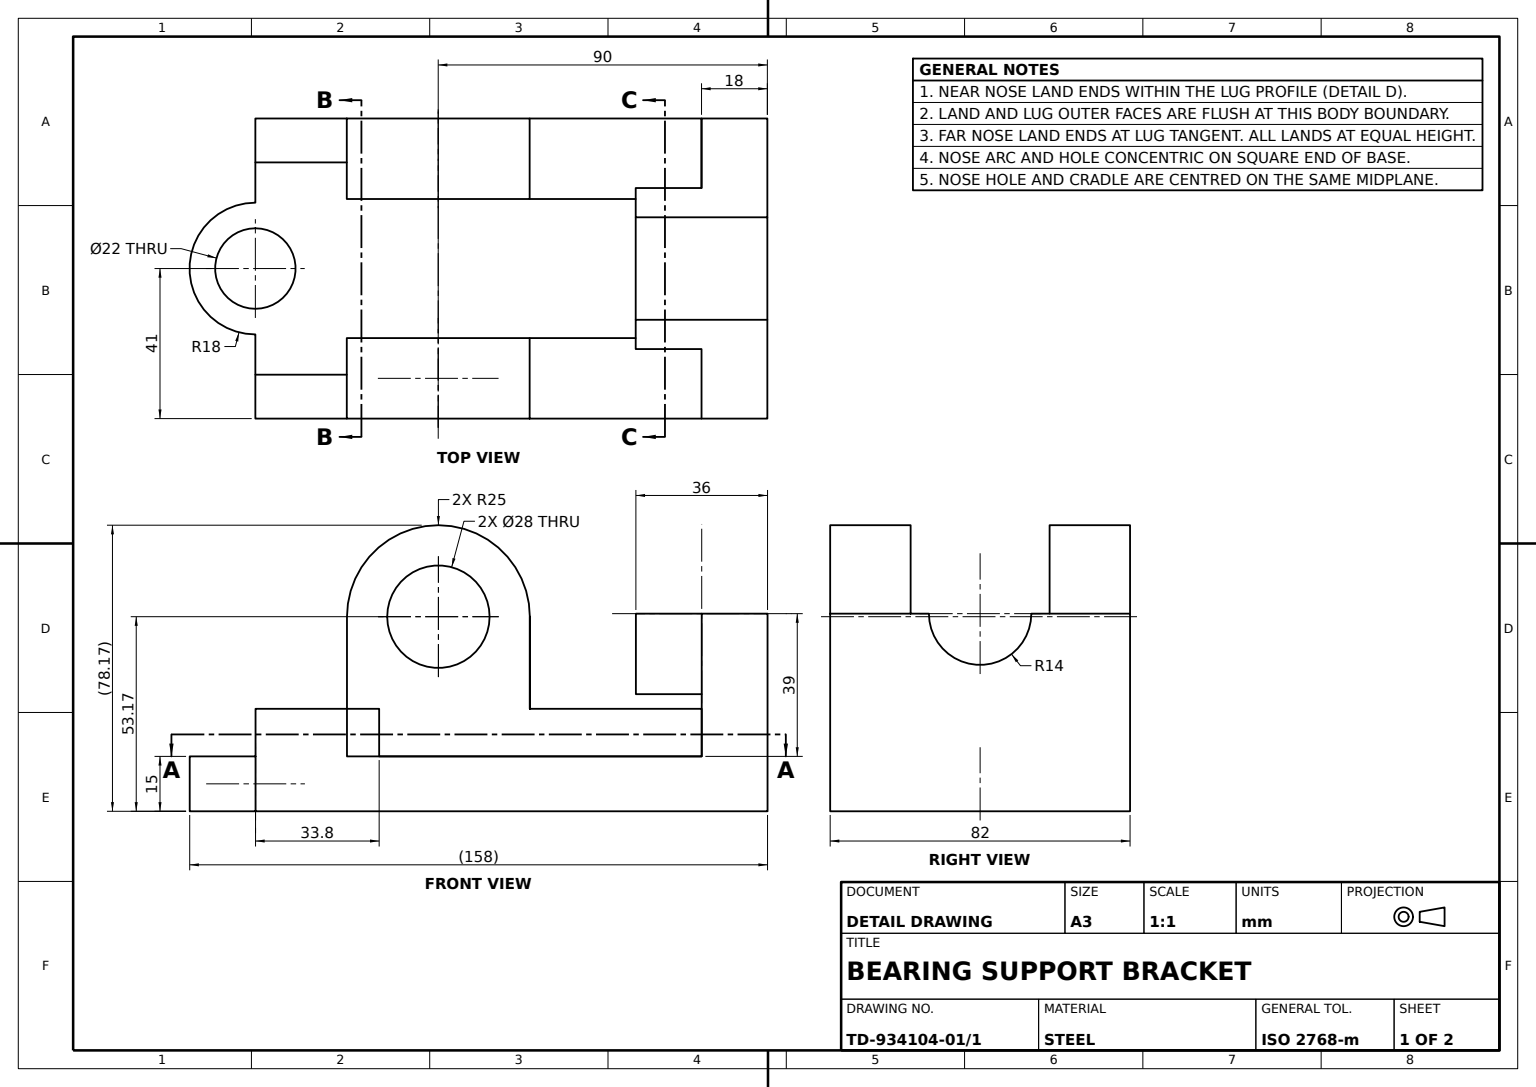
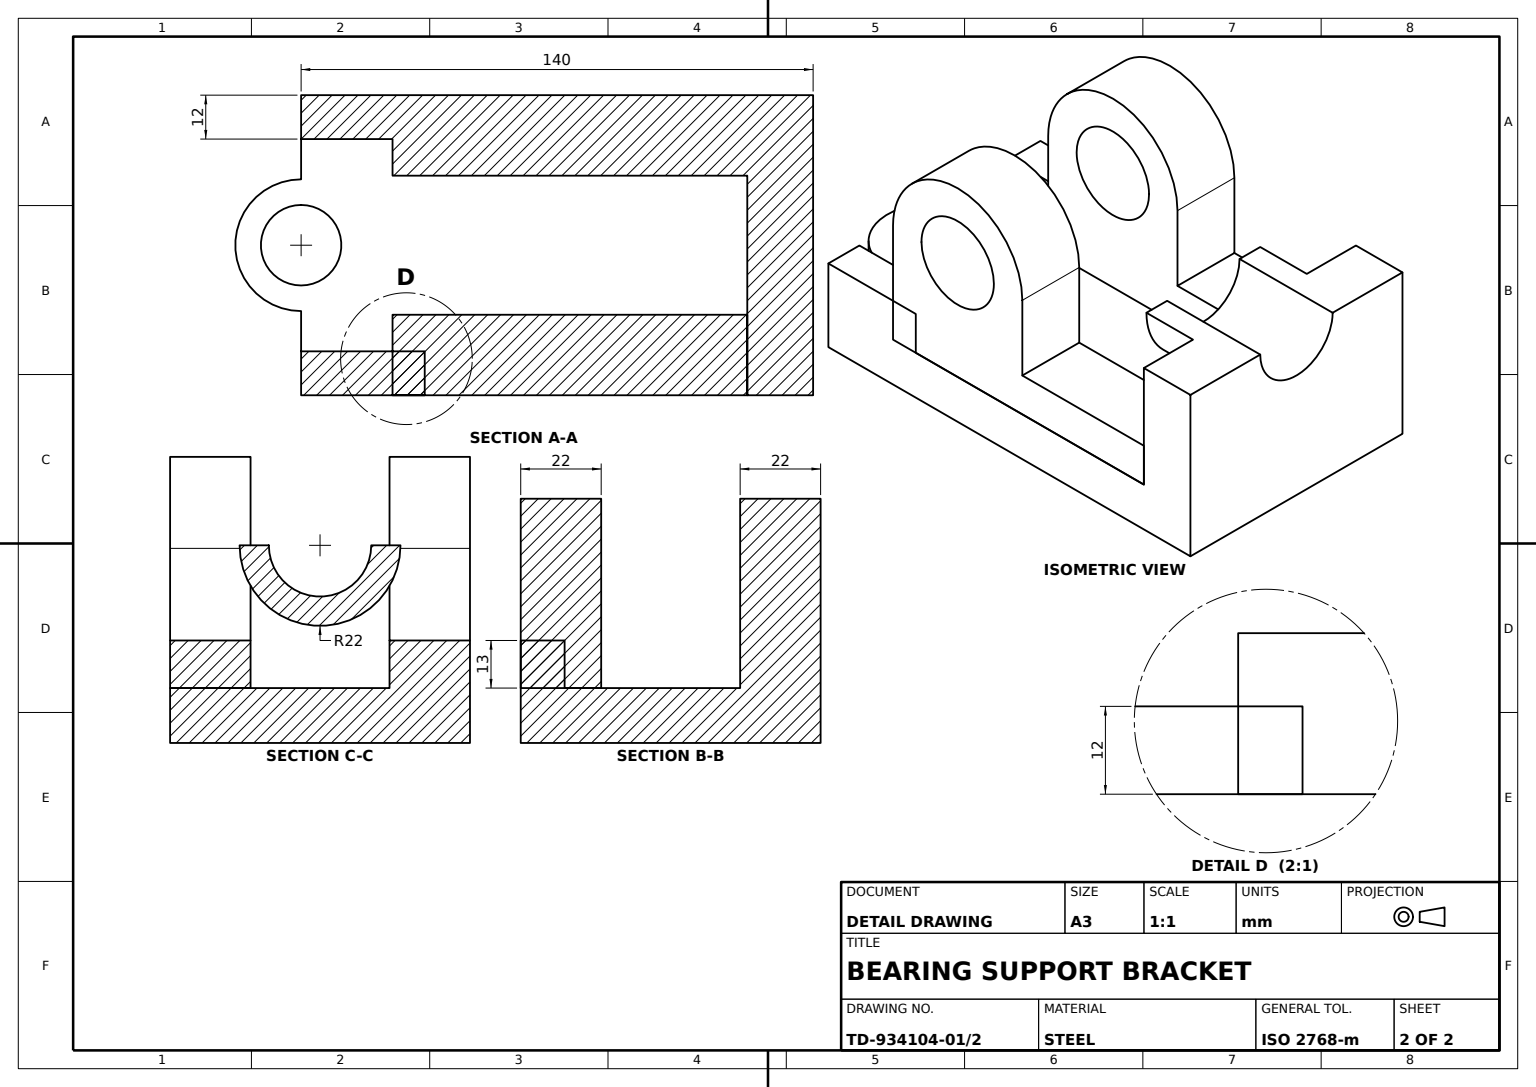
SolidWorks part; units mm, degrees
material "Plain Carbon Steel"
ref_plane "Front Plane" through (0, 0, 0) normal (0, 0, 1) x (1, 0, 0)
ref_plane "Top Plane" through (0, 0, 0) normal (0, 1, 0) x (1, 0, 0)
ref_plane "Right Plane" through (0, 0, 0) normal (1, 0, 0) x (0, 0, -1)
sketch "Base Plate Sketch" plane through (0, 0, 0) normal (0, 1, 0) x (1, 0, 0)
  line L1 (-70, 41) -> (70, 41)
  line L2 (-70, 41) -> (-70, -41)
  line L3 (-70, -41) -> (70, -41)
  line L4 (70, 41) -> (70, -41)
  line L5 (-70, 41) -> (70, -41) construction
  line L6 (-70, -41) -> (70, 41) construction
  point P0 (0, 0)
  dimension "D1" = 140
  dimension "D2" = 82
extrude "Base Plate 140x82x15" add sketch "Base Plate Sketch" along normal mid plane 15
sketch "Side Wall Sketch" plane through (0, 7.5, 0) normal (0, 1, 0) x (1, 0, 0)
  line L0 (-70, -41) -> (70, -41) construction
  line L1 (70, 41) -> (52, 41)
  line L2 (70, 41) -> (70, -41)
  line L3 (70, -41) -> (52, -41)
  line L4 (52, 41) -> (52, -41)
  dimension "D1" = 18
extrude "Side Wall" add sketch "Side Wall Sketch" along normal blind 39
sketch "Wall Extension Sketch" plane through (52, 0, 0) normal (-1, 0, 0) x (0, 0, 1)
  line L0 (-41, 46.5) -> (41, 46.5) construction
  line L1 (-22, 46.5) -> (22, 46.5)
  arc A0 (-14, 46.5) -> (14, 46.5) centre (0, 46.5) ccw
  arc A1 (-22, 46.5) -> (22, 46.5) centre (0, 46.5) ccw
  line M5 (41, 46.5) -> (-41, 46.5)
  dimension "D1" = 14
  dimension "D2" = 22
extrude "Wall Extension" add sketch "Wall Extension Sketch" along normal blind 18 contours A1 A0 M5
sketch "Wall Slot Sketch" plane through (70, 0, 0) normal (1, 0, 0) x (0, 0, -1)
  line L0 (-41, 46.5) -> (41, 46.5) construction
  line L1 (-14, 46.5) -> (14, 46.5)
  arc A0 (-14, 46.5) -> (14, 46.5) centre (0, 46.5) ccw
extrude "Wall Slot Cut" cut sketch "Wall Slot Sketch" against normal blind 18
sketch "End Block Sketch" plane through (0, 7.5, 0) normal (0, 1, 0) x (1, 0, 0)
  line L1 (-70, -41) -> (-36.2, -41)
  line L2 (-70, -41) -> (-70, -29)
  line L3 (-70, -29) -> (-36.2, -29)
  line L4 (-36.2, -41) -> (-36.2, -29)
  line L6 (-70, -38.5363) -> (-70, -37.0533)
  line L7 (52, 41) -> (-70, 41) construction
  line M4 (-70, 41) -> (-70, -41)
  line M5 (-70, -41) -> (52, -41)
  dimension "D1" = 12
  dimension "D2" = 78.0533
  dimension "33.8" = 33.8
  dimension "D3" = 79.5363
extrude "End Block" add sketch "End Block Sketch" along normal blind 13 contours L4 L3 L2 M5 M4
sketch "Bearing Lug Sketch" plane through (0, 0, 41) normal (0, 0, 1) x (1, 0, 0)
  line L0 (70, 46.5) -> (70, -7.5) construction
  line L1 (-45, 45.6685) -> (-45, 7.5)
  line L2 (-36.2, 7.5) -> (52, 7.5) construction
  line L3 (5, 45.6685) -> (5, 20.5)
  line L4 (5, 20.5) -> (52, 20.5)
  line L5 (-70, -7.5) -> (70, -7.5) construction
  line L6 (52, 46.5) -> (52, 7.5) construction
  line L15 (-70, -7.5) -> (70, -7.5)
  line L16 (70, -7.5) -> (70, 46.5)
  line L17 (70, 46.5) -> (52, 46.5)
  line L18 (52, 46.5) -> (52, 7.5)
  line L19 (52, 7.5) -> (-36.2, 7.5)
  line L20 (-36.2, 7.5) -> (-36.2, 20.5)
  line L21 (-36.2, 20.5) -> (-70, 20.5)
  line L22 (-70, 20.5) -> (-70, -7.5)
  line L26 (52, 20.5) -> (52, 7.5)
  line L27 (52, 7.5) -> (-45, 7.5)
  arc A1 (5, 45.6685) -> (-45, 45.6685) centre (-20, 45.6685) ccw
  dimension "D1" = 90
  dimension "D4" = 25
  dimension "D2" = 28
  dimension "D5" = 53.1685
  dimension "D3" = 0
extrude "Bearing Lug" add sketch "Bearing Lug Sketch" against normal blind 22 separate body
ref_plane "Plane5" through (0, 0, 0) normal (0, 0, 1) x (1, 0, 0)
mirror "Bearing Lug Mirror" about plane through (0, 0, 0) normal (0, 0, 1) of "Bearing Lug"
mirror "End Block Mirror" about plane through (0, 0, 0) normal (0, 0, 1) of "End Block"
sketch "Lug Bore Sketch" plane through (0, 0, 41) normal (0, 0, 1) x (1, 0, 0)
  circle A0 centre (-20, 45.6685) radius 14
  dimension "D1" = 28
extrude "Lug Bore" cut sketch "Lug Bore Sketch" against normal through all both and the other way through all
sketch "Cradle Boss Sketch" plane through (0, 7.5, 0) normal (0, 1, 0) x (1, 0, 0)
  line L0 (-70, 29) -> (-70, -29) construction
  circle A0 centre (-70, 0) radius 18
  dimension "D1" = 36
extrude "Cradle Boss" add sketch "Cradle Boss Sketch" against normal blind 15
sketch "Cradle Sketch" plane through (0, 7.5, 0) normal (0, 1, 0) x (1, 0, 0)
  circle A0 centre (-70, 0) radius 11
  dimension "D1" = 22
extrude "Cradle Cut" cut sketch "Cradle Sketch" against normal blind 15
